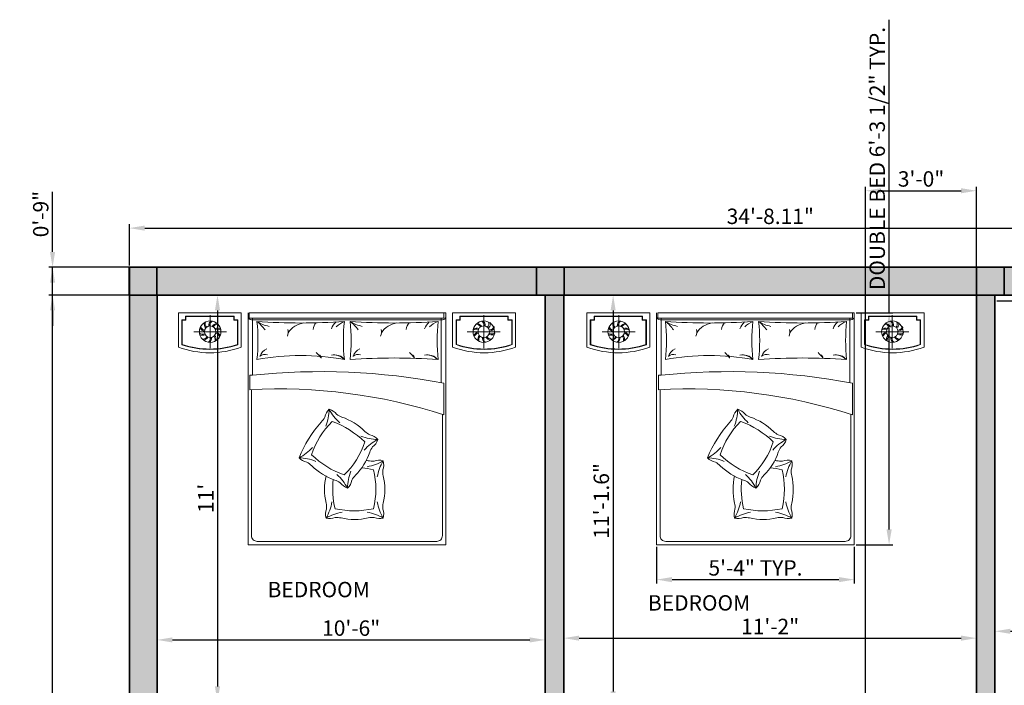
# Model space of a CAD drawing. Units: inches. Extents: x -36 to 490, y -420 to 94.
# Tile 3 of 4: x -36 to 284, y -122 to 94. Entities that reach past the tile are written whole.
import ezdxf

# ---------------------------------------------------------------- set-up
doc = ezdxf.new("R2010")
doc.units = ezdxf.units.IN
for name, color, linetype, lineweight in [('A-ANNO-DIMS', 2, 'Continuous', 18), ('A-AREA-IDEN', 1, 'Continuous', 18), ('A-COLS', 1, 'Continuous', 35), ('A-WALL', 7, 'Continuous', 35), ('furn', 8, 'Continuous', 18)]:
    doc.layers.add(name, color=color, linetype=linetype, lineweight=lineweight)
doc.layers.add('A-WALL-PATT', color=177, linetype='Continuous', lineweight=13, true_color=0x293189)
doc.styles.get("Standard").update_dxf_attribs({"font": 'arial.ttf'})
doc.dimstyles.new('ISO-25', dxfattribs={"dimtxt": 5, "dimasz": 5, "dimexe": 1.25, "dimexo": 0.625, "dimtad": 1, "dimlunit": 3, "dimtxsty": 'Standard', "dimcen": 2.5, "dimadec": 0, "dimazin": 0, "dimtfac": 1, "dimtmove": 0, "dimatfit": 3, "dimfxl": 1, "dimarcsym": 0})

# ---------------------------------------------------------------- blocks, each defined once
blk = doc.blocks.new('*D11')
at = {"layer": 'A-ANNO-DIMS', "color": 0, "lineweight": -2, "transparency": 16777216}
for p, q in [((8.98, -106.51), (8.98, -105.89)), ((13.98, -107.14), (129.98, -107.14)), ((134.98, -106.51), (134.98, -105.89))]:
    blk.add_line(p, q, dxfattribs=at)
at = {"layer": 'A-ANNO-DIMS', "color": 0, "transparency": 16777216}
for points in [[(13.98, -106.3), (13.98, -107.97), (8.98, -107.14)], [(129.98, -106.3), (129.98, -107.97), (134.98, -107.14)]]:
    blk.add_solid(points, dxfattribs=at)
at = {"layer": 'Defpoints', "color": 0, "transparency": 16777216}
for p in [(8.98, -107.14), (134.98, -107.14), (134.98, -107.14)]:
    blk.add_point(p, dxfattribs=at)
at = {"layer": 'A-ANNO-DIMS', "color": 0, "transparency": 16777216, "insert": (71.98, -103.96), "char_height": 5, "attachment_point": 5}
blk.add_mtext('10\'-6"', dxfattribs=at)
blk = doc.blocks.new('*D12')
at = {"layer": 'A-ANNO-DIMS', "color": 0, "lineweight": -2, "transparency": 16777216}
for p, q in [((9.61, 4.77), (29.84, 4.77)), ((28.59, -0.23), (28.59, -122.23)), ((9.61, -127.23), (29.84, -127.23))]:
    blk.add_line(p, q, dxfattribs=at)
at = {"layer": 'A-ANNO-DIMS', "color": 0, "transparency": 16777216}
for points in [[(27.76, -0.23), (29.43, -0.23), (28.59, 4.77)], [(27.76, -122.23), (29.43, -122.23), (28.59, -127.23)]]:
    blk.add_solid(points, dxfattribs=at)
at = {"layer": 'Defpoints', "color": 0, "transparency": 16777216}
for p in [(8.98, 4.77), (8.98, -127.23), (28.59, -127.23)]:
    blk.add_point(p, dxfattribs=at)
at = {"layer": 'A-ANNO-DIMS', "color": 0, "transparency": 16777216, "insert": (25.46, -61.23), "char_height": 5, "attachment_point": 5, "rotation": 90}
blk.add_mtext("11'", dxfattribs=at)
blk = doc.blocks.new('*D13')
at = {"layer": 'A-ANNO-DIMS', "color": 0, "lineweight": -2, "transparency": 16777216}
for p, q in [((140.98, -105.94), (140.98, -105.31)), ((274.98, -105.94), (274.98, -105.31)), ((145.98, -106.56), (269.98, -106.56))]:
    blk.add_line(p, q, dxfattribs=at)
at = {"layer": 'A-ANNO-DIMS', "color": 0, "transparency": 16777216}
for points in [[(145.98, -105.73), (145.98, -107.39), (140.98, -106.56)], [(269.98, -105.73), (269.98, -107.39), (274.98, -106.56)]]:
    blk.add_solid(points, dxfattribs=at)
at = {"layer": 'Defpoints', "color": 0, "transparency": 16777216}
for p in [(140.98, -106.56), (274.98, -106.56), (274.98, -106.56)]:
    blk.add_point(p, dxfattribs=at)
at = {"layer": 'A-ANNO-DIMS', "color": 0, "transparency": 16777216, "insert": (207.98, -103.42), "char_height": 5, "attachment_point": 5}
blk.add_mtext('11\'-2"', dxfattribs=at)
blk = doc.blocks.new('*D14')
at = {"layer": 'A-ANNO-DIMS', "color": 0, "lineweight": -2, "transparency": 16777216}
for p, q in [((141.61, 4.77), (158.28, 4.77)), ((157.03, -0.23), (157.03, -123.83)), ((143.3, -128.83), (158.28, -128.83))]:
    blk.add_line(p, q, dxfattribs=at)
at = {"layer": 'A-ANNO-DIMS', "color": 0, "transparency": 16777216}
for points in [[(156.2, -0.23), (157.86, -0.23), (157.03, 4.77)], [(156.2, -123.83), (157.86, -123.83), (157.03, -128.83)]]:
    blk.add_solid(points, dxfattribs=at)
at = {"layer": 'Defpoints', "color": 0, "transparency": 16777216}
for p in [(140.98, 4.77), (142.67, -128.83), (157.03, -128.83)]:
    blk.add_point(p, dxfattribs=at)
at = {"layer": 'A-ANNO-DIMS', "color": 0, "transparency": 16777216, "insert": (153.85, -62.03), "char_height": 5, "attachment_point": 5, "rotation": 90}
blk.add_mtext('11\'-1.6"', dxfattribs=at)
blk = doc.blocks.new('*D15')
at = {"layer": 'A-ANNO-DIMS', "color": 0, "lineweight": -2, "transparency": 16777216}
for p, q in [((281.61, 2.85), (295.66, 2.85)), ((294.41, -2.15), (294.41, -122.23)), ((281.61, -127.23), (295.66, -127.23))]:
    blk.add_line(p, q, dxfattribs=at)
at = {"layer": 'A-ANNO-DIMS', "color": 0, "transparency": 16777216}
for points in [[(293.58, -2.15), (295.25, -2.15), (294.41, 2.85)], [(293.58, -122.23), (295.25, -122.23), (294.41, -127.23)]]:
    blk.add_solid(points, dxfattribs=at)
at = {"layer": 'Defpoints', "color": 0, "transparency": 16777216}
for p in [(280.98, 2.85), (280.98, -127.23), (294.41, -127.23)]:
    blk.add_point(p, dxfattribs=at)
at = {"layer": 'A-ANNO-DIMS', "color": 0, "transparency": 16777216, "insert": (291.24, -62.19), "char_height": 5, "attachment_point": 5, "rotation": 90}
blk.add_mtext('10\'-10.08"', dxfattribs=at)
blk = doc.blocks.new('*D16')
at = {"layer": 'A-ANNO-DIMS', "color": 0, "lineweight": -2, "transparency": 16777216}
for p, q in [((280.98, -103.71), (280.98, -103.08)), ((285.98, -104.33), (401.98, -104.33)), ((406.98, -103.71), (406.98, -103.08))]:
    blk.add_line(p, q, dxfattribs=at)
at = {"layer": 'A-ANNO-DIMS', "color": 0, "transparency": 16777216}
for points in [[(285.98, -103.5), (285.98, -105.17), (280.98, -104.33)], [(401.98, -103.5), (401.98, -105.17), (406.98, -104.33)]]:
    blk.add_solid(points, dxfattribs=at)
at = {"layer": 'Defpoints', "color": 0, "transparency": 16777216}
for p in [(280.98, -104.33), (406.98, -104.33), (406.98, -104.33)]:
    blk.add_point(p, dxfattribs=at)
at = {"layer": 'A-ANNO-DIMS', "color": 0, "transparency": 16777216, "insert": (343.98, -101.16), "char_height": 5, "attachment_point": 5}
blk.add_mtext('10\'-6"', dxfattribs=at)
blk = doc.blocks.new('*D21')
at = {"layer": 'A-ANNO-DIMS', "color": 0, "lineweight": -2, "transparency": 16777216}
for p, q in [((-0.02, 14.4), (-0.02, 27.74)), ((4.98, 26.49), (411.1, 26.49)), ((416.1, 14.4), (416.1, 27.74))]:
    blk.add_line(p, q, dxfattribs=at)
at = {"layer": 'A-ANNO-DIMS', "color": 0, "transparency": 16777216}
for points in [[(4.98, 27.33), (4.98, 25.66), (-0.02, 26.49)], [(411.1, 27.33), (411.1, 25.66), (416.1, 26.49)]]:
    blk.add_solid(points, dxfattribs=at)
at = {"layer": 'Defpoints', "color": 0, "transparency": 16777216}
for p in [(416.1, 26.49), (-0.02, 13.77), (416.1, 13.77)]:
    blk.add_point(p, dxfattribs=at)
at = {"layer": 'A-ANNO-DIMS', "color": 0, "transparency": 16777216, "insert": (208.04, 29.67), "char_height": 5, "attachment_point": 5}
blk.add_mtext('34\'-8.11"', dxfattribs=at)
blk = doc.blocks.new('BED-DOUBLE')
for p, q in [((1.43, 73.57), (1.43, 55.04)), ((62.71, 73.57), (62.71, 52.63)), ((1.11, 73.01), (63.06, 73.01))]:
    blk.add_line(p, q)
for points in [[(0, 75.3), (0, 0), (64.18, 0), (64.18, 75.3)], [(63.58, 75.3), (63.58, 73.57), (0.37, 73.57), (0.37, 75.3), (64.18, 75.3)]]:
    blk.add_lwpolyline(points)
for points in [[(2.84, 60.1, 0.058596), (2.84, 72.5, 0.036889), (31.25, 72.5, 0.052163), (31.25, 60.1, 0.093111)], [(33.1, 60.1, 0.058596), (33.1, 72.5, 0.036648), (61.69, 72.5, 0.052163), (61.69, 60.1, 0.036967)], [(0.56, 55.04), (1.43, 55.04, -0.072944), (63.58, 52.45), (63.58, 42.16, 0.092568), (0.56, 50.32)]]:
    blk.add_lwpolyline(points, format="xyb", close=True)
for points in [[(1.11, 50.35), (1.11, 2.97, 0.414214), (2.97, 1.11), (61.21, 1.11, 0.414214), (63.06, 2.97), (63.06, 42.34)], [(25.2, 38.53, 0.091296), (26.33, 43.97, 0.091296), (29.75, 39.6, 0.091296)], [(20.61, 29.25, 0.111006), (31.2, 22.66, 0.119549), (37.88, 33.38, 0.107813), (27.32, 40)], [(27.26, 39.98, 0.121865), (20.61, 29.25, 0.121865)], [(36.64, 35.3, 0.091296), (42.07, 34.16, 0.091296), (37.69, 30.75, 0.091296)], [(32.26, 18.42, 0.159461), (33.7, 20.96, -0.076283), (34.84, 22.55, 0.115075), (39.49, 30.02, -0.076283), (40.42, 31.75, 0.159461), (42.07, 34.16)], [(21.95, 27.08, 0.091296), (16.52, 28.23, 0.091296), (20.9, 31.63, 0.091296)], [(38.64, 25.34, 0.091296), (43.86, 27.24, 0.091296), (41.94, 22.03, 0.091296)], [(43.86, 8.69, 0.159461), (43.73, 11.61, -0.076283), (43.86, 13.56, 0.115075), (43.86, 22.37, -0.076283), (43.73, 24.32, 0.159461), (43.86, 27.24)], [(28.24, 11.72, 0.111006), (40.71, 11.73, 0.119549), (40.71, 24.36, 0.033212), (36.88, 24.95)], [(33.39, 23.85, 0.091296), (32.26, 18.42, 0.091296), (28.84, 22.79)], [(30.52, 10.59, 0.091296), (25.31, 8.69, 0.091296), (27.23, 13.9, 0.091296)], [(41.94, 13.9, 0.091296), (43.86, 8.69, 0.091296), (38.64, 10.59)]]:
    blk.add_lwpolyline(points, format="xyb")
for centre, radius, start, end in [((1.11, 74.12), 1.11, 180, 270), ((63.06, 74.12), 1.11, 270, 0), ((9.44, 82.87), 12.28, 237.5379, 257.5233), ((-6.45, 60.91), 14.86, 36.4935, 51.2792), ((18.86, 65.15), 6.88, 96.6849, 148.3182), ((25.81, 69.06), 4.82, 141.8174, 169.8987), ((31.91, 68.38), 5.19, 130.5354, 160.3558), ((35.15, 64), 9.35, 114.6457, 134.1585), ((23.8, 60.91), 14.86, 36.4935, 51.2792), ((39.69, 82.87), 12.28, 237.5379, 257.5233), ((49.11, 65.15), 6.88, 96.6849, 148.3182), ((56.06, 69.06), 4.82, 141.8174, 169.8987), ((62.16, 68.38), 5.19, 130.5354, 160.3558), ((65.4, 64), 9.35, 114.6457, 134.1585), ((9.94, 68.98), 3.08, 335.8927, 16.1192), ((40.19, 68.98), 3.08, 335.8927, 16.1192), ((7.73, 59.82), 4.12, 114.2916, 160.9896), ((5.59, 58.96), 2.82, 76.4823, 128.5563), ((11.2, 51.48), 15.49, 36.2085, 45.0849), ((22.66, 60.63), 1.04, 353.7543, 77.2187), ((27.63, 56.56), 5.07, 44.406, 96.8342), ((28.58, 58.33), 3.21, 33.6349, 90.8456), ((37.98, 59.82), 4.12, 114.2916, 160.9896), ((35.84, 58.96), 2.82, 76.4823, 128.5563), ((41.46, 51.48), 15.49, 36.2085, 45.0849), ((52.91, 60.63), 1.04, 353.7543, 77.2187), ((57.88, 56.56), 5.07, 44.406, 96.8342), ((58.83, 58.33), 3.21, 33.6349, 90.8456), ((29.5, 40.5), 4.7, 132.4658, 168.7065), ((25.09, 39.6), 4.54, 37.2937, 74.0973), ((32.54, 47.52), 6.44, 233.2983, 250.7472), ((54.12, 12.85), 40.62, 138.3818, 157.7644), ((19.15, 44.34), 6.44, 315.5854, 333.0343), ((24.23, 23.07), 19.38, 45.1307, 71.3884), ((42.4, 41.42), 6.44, 225.7718, 243.2208), ((38.72, 31.4), 4.34, 39.4726, 79.6505), ((19.98, 31.41), 4.7, 222.6522, 258.8929), ((16.17, 21.05), 6.44, 45.7718, 63.2208), ((34.34, 39.4), 19.38, 225.1307, 251.3884), ((34.58, 8.4), 19.38, 77.0576, 78.7033), ((40.3, 33.58), 6.44, 257.6988, 275.1477), ((42.47, 23.13), 4.34, 71.3996, 111.5774), ((44.18, 17.97), 19.38, 166.8711, 193.1289), ((53.75, 18.1), 26.29, 173.1956, 194.0284), ((26.03, 14.95), 6.44, 53.2983, 70.7472), ((34.07, 23.48), 5.38, 218.7754, 250.3571), ((19.02, 12.17), 6.44, 355.0387, 12.4877), ((29.84, 9.96), 4.7, 159.3666, 195.6073), ((26.56, 13.23), 4.7, 254.5791, 290.8198), ((28.81, 2.42), 6.44, 77.6988, 95.1477), ((34.52, 27.6), 19.38, 257.0576, 283.3153), ((40.4, 2.45), 6.44, 85.2252, 102.6741), ((42.71, 13.95), 5.38, 250.7023, 282.284)]:
    blk.add_arc(centre, radius, start, end)
blk = doc.blocks.new('NIGHTSTAND-LAMP-L')
for p, q in [((10.31, 1.49), (10.31, 12.19)), ((4.96, 6.84), (15.66, 6.84))]:
    blk.add_line(p, q)
blk.add_lwpolyline([(0, 1.86), (0, 12.98), (20.4, 12.98), (20.4, 1.86, -0.181818)], format="xyb", close=True)
for points in [[(2.34, 11.87), (2.34, 10.65), (1.11, 10.65)], [(2.45, 11.87), (2.45, 10.54), (1.11, 10.54)], [(2.34, 11.87), (18.07, 11.87)], [(2.34, 11.76), (18.07, 11.76)], [(17.95, 11.87), (17.95, 10.54), (19.29, 10.54)], [(18.07, 11.87), (18.07, 10.65), (19.29, 10.65)]]:
    blk.add_lwpolyline(points)
for points in [[(19.29, 10.65), (19.29, 2.63, -0.167087), (1.11, 2.63), (1.11, 10.65)], [(19.18, 10.65), (19.18, 2.71, -0.165559), (1.22, 2.71), (1.22, 10.65)]]:
    blk.add_lwpolyline(points, format="xyb")
for radius in [3.49, 1.89]:
    blk.add_circle((10.31, 6.84), radius)
for centre, radius, start, end in [((10.62, 9.46), 2.24, 172.17, 218.4897), ((10.4, 9.41), 1.71, 160.3002, 220.538), ((12.1, 8.78), 2.24, 136.17, 182.4897), ((11.89, 8.87), 1.71, 124.3002, 184.538), ((9.02, 9.14), 2.24, 208.17, 254.4897), ((8.87, 8.97), 1.71, 196.3002, 256.538), ((12.89, 7.36), 2.24, 100.17, 146.4897), ((12.78, 7.55), 1.71, 88.3002, 148.538), ((12.7, 5.74), 2.24, 64.17, 110.4897), ((12.72, 5.96), 1.71, 52.3002, 112.538), ((11.59, 4.54), 2.24, 28.17, 74.4897), ((7.89, 7.72), 1.71, 232.3002, 292.538), ((7.91, 7.94), 2.24, 244.17, 290.4897), ((7.84, 6.13), 1.71, 268.3002, 328.538), ((7.72, 6.33), 2.24, 280.17, 326.4897), ((8.72, 4.82), 1.71, 304.3002, 4.538), ((8.52, 4.9), 2.24, 316.17, 2.4897), ((10.22, 4.27), 1.71, 340.3002, 40.538), ((10, 4.22), 2.24, 352.17, 38.4897), ((11.74, 4.71), 1.71, 16.3002, 76.538)]:
    blk.add_arc(centre, radius, start, end)
blk = doc.blocks.new('NIGHTSTAND-LAMP-R')
for p, q in [((10.1, 1.49), (10.1, 12.18)), ((15.45, 6.83), (4.75, 6.83))]:
    blk.add_line(p, q)
blk.add_lwpolyline([(20.4, 1.85), (20.4, 12.98), (0, 12.98), (0, 1.85, 0.181818)], format="xyb", close=True)
for points in [[(2.34, 11.87), (2.34, 10.65), (1.11, 10.65)], [(2.45, 11.87), (2.45, 10.53), (1.11, 10.53)], [(18.07, 11.87), (2.34, 11.87)], [(18.07, 11.76), (2.34, 11.76)], [(17.95, 11.87), (17.95, 10.53), (19.29, 10.53)], [(18.07, 11.87), (18.07, 10.65), (19.29, 10.65)]]:
    blk.add_lwpolyline(points)
for points in [[(1.11, 10.65), (1.11, 2.63, 0.167087), (19.29, 2.63), (19.29, 10.65)], [(1.22, 10.65), (1.22, 2.71, 0.165559), (19.18, 2.71), (19.18, 10.65)]]:
    blk.add_lwpolyline(points, format="xyb")
for radius in [3.49, 1.89]:
    blk.add_circle((10.1, 6.83), radius)
for centre, radius, start, end in [((8.51, 8.86), 1.71, 355.462, 55.6998), ((8.31, 8.77), 2.24, 357.5103, 43.83), ((10.01, 9.4), 1.71, 319.462, 19.6998), ((10.04, 9.55), 2.24, 321.5103, 7.83), ((7.68, 5.95), 1.71, 67.462, 127.6998), ((7.7, 5.73), 2.24, 69.5103, 115.83), ((8.81, 4.54), 2.24, 105.5103, 151.83), ((7.62, 7.54), 1.71, 31.462, 91.6998), ((7.51, 7.35), 2.24, 33.5103, 79.83), ((12.77, 7.81), 1.71, 247.462, 307.6998), ((11.79, 9.06), 1.71, 283.462, 343.6998), ((11.64, 9.23), 2.24, 285.5103, 331.83), ((8.66, 4.7), 1.71, 103.462, 163.6998), ((10.41, 4.22), 2.24, 141.5103, 187.83), ((10.19, 4.27), 1.71, 139.462, 199.6998), ((11.88, 4.9), 2.24, 177.5103, 223.83), ((11.68, 4.81), 1.71, 175.462, 235.6998), ((12.68, 6.32), 2.24, 213.5103, 259.83), ((12.57, 6.13), 1.71, 211.462, 271.6998), ((12.74, 8.03), 2.24, 249.5103, 295.83)]:
    blk.add_arc(centre, radius, start, end)
blk = doc.blocks.new('COLUMN-9X9')
h = blk.add_hatch(color=256)
h.dxf.hatch_style = 1
h.paths.add_polyline_path([(9, 0), (9, 9), (0, 9), (0, 0)])
blk.add_lwpolyline([(0, 9), (9, 9), (9, 0), (0, 0)], close=True)
blk = doc.blocks.new('*D30')
at = {"layer": 'A-ANNO-DIMS', "color": 0, "lineweight": -2, "transparency": 16777216}
for p, q in [((246.61, -0.97), (246.61, 94.12)), ((235.94, -0.97), (247.86, -0.97)), ((246.61, -71.28), (246.61, -5.97)), ((235.94, -76.28), (247.86, -76.28))]:
    blk.add_line(p, q, dxfattribs=at)
at = {"layer": 'A-ANNO-DIMS', "color": 0, "transparency": 16777216}
for points in [[(245.78, -5.97), (247.45, -5.97), (246.61, -0.97)], [(245.78, -71.28), (247.45, -71.28), (246.61, -76.28)]]:
    blk.add_solid(points, dxfattribs=at)
at = {"layer": 'Defpoints', "color": 0, "transparency": 16777216}
for p in [(235.32, -0.97), (246.61, -0.97), (235.32, -76.28)]:
    blk.add_point(p, dxfattribs=at)
at = {"layer": 'A-ANNO-DIMS', "color": 0, "transparency": 16777216, "insert": (243.4, 49.07), "char_height": 5, "attachment_point": 5, "rotation": 90}
blk.add_mtext('DOUBLE BED 6\'-3 1/2" TYP.', dxfattribs=at)
blk = doc.blocks.new('*D31')
at = {"layer": 'A-ANNO-DIMS', "color": 0, "lineweight": -2, "transparency": 16777216}
for p, q in [((171.14, -76.9), (171.14, -88.82)), ((235.32, -76.9), (235.32, -88.82)), ((176.14, -87.57), (230.32, -87.57))]:
    blk.add_line(p, q, dxfattribs=at)
at = {"layer": 'A-ANNO-DIMS', "color": 0, "transparency": 16777216}
for points in [[(176.14, -86.74), (176.14, -88.41), (171.14, -87.57)], [(230.32, -86.74), (230.32, -88.41), (235.32, -87.57)]]:
    blk.add_solid(points, dxfattribs=at)
at = {"layer": 'Defpoints', "color": 0, "transparency": 16777216}
for p in [(171.14, -76.28), (235.32, -76.28), (235.32, -87.57)]:
    blk.add_point(p, dxfattribs=at)
at = {"layer": 'A-ANNO-DIMS', "color": 0, "transparency": 16777216, "insert": (203.23, -84.41), "char_height": 5, "attachment_point": 5}
blk.add_mtext('5\'-4" TYP.', dxfattribs=at)
blk = doc.blocks.new('*D39')
at = {"layer": 'A-ANNO-DIMS', "color": 0, "lineweight": -2, "transparency": 16777216}
for p, q in [((238.98, -244.38), (238.98, 39.87)), ((243.98, 38.62), (269.98, 38.62)), ((274.98, -244.38), (274.98, 39.87))]:
    blk.add_line(p, q, dxfattribs=at)
at = {"layer": 'A-ANNO-DIMS', "color": 0, "transparency": 16777216}
for points in [[(243.98, 39.45), (243.98, 37.79), (238.98, 38.62)], [(269.98, 39.45), (269.98, 37.79), (274.98, 38.62)]]:
    blk.add_solid(points, dxfattribs=at)
at = {"layer": 'Defpoints', "color": 0, "transparency": 16777216}
for p in [(274.98, 38.62), (238.98, -245.01), (274.98, -245.01)]:
    blk.add_point(p, dxfattribs=at)
at = {"layer": 'A-ANNO-DIMS', "color": 0, "transparency": 16777216, "insert": (256.98, 41.8), "char_height": 5, "attachment_point": 5}
blk.add_mtext('3\'-0"', dxfattribs=at)
blk = doc.blocks.new('*D42')
at = {"layer": 'A-ANNO-DIMS', "color": 0, "lineweight": -2, "transparency": 16777216}
for p, q in [((-0.64, 13.77), (-26.2, 13.77)), ((-24.95, -385.69), (-24.95, 8.77)), ((140.36, -390.69), (-26.2, -390.69))]:
    blk.add_line(p, q, dxfattribs=at)
at = {"layer": 'A-ANNO-DIMS', "color": 0, "transparency": 16777216}
for points in [[(-25.78, 8.77), (-24.12, 8.77), (-24.95, 13.77)], [(-25.78, -385.69), (-24.12, -385.69), (-24.95, -390.69)]]:
    blk.add_solid(points, dxfattribs=at)
at = {"layer": 'Defpoints', "color": 0, "transparency": 16777216}
for p in [(-24.95, 13.77), (-0.02, 13.77), (140.98, -390.69)]:
    blk.add_point(p, dxfattribs=at)
at = {"layer": 'A-ANNO-DIMS', "color": 0, "transparency": 16777216, "insert": (-28.16, -188.46), "char_height": 5, "attachment_point": 5, "rotation": 90}
blk.add_mtext('33\'-8 1/2"', dxfattribs=at)
blk = doc.blocks.new('*D50')
at = {"layer": 'A-ANNO-DIMS', "color": 0, "lineweight": -2, "transparency": 16777216}
for p, q in [((-24.95, 18.77), (-24.95, 38.31)), ((8.28, 13.77), (-26.2, 13.77)), ((-24.95, 4.77), (-24.95, 13.77)), ((8.36, 4.77), (-26.2, 4.77)), ((-24.95, -0.23), (-24.95, -5.23))]:
    blk.add_line(p, q, dxfattribs=at)
at = {"layer": 'A-ANNO-DIMS', "color": 0, "transparency": 16777216}
for points in [[(-25.78, 18.77), (-24.12, 18.77), (-24.95, 13.77)], [(-25.78, -0.23), (-24.12, -0.23), (-24.95, 4.77)]]:
    blk.add_solid(points, dxfattribs=at)
at = {"layer": 'Defpoints', "color": 0, "transparency": 16777216}
for p in [(-24.95, 13.77), (8.9, 13.77), (8.98, 4.77)]:
    blk.add_point(p, dxfattribs=at)
at = {"layer": 'A-ANNO-DIMS', "color": 0, "transparency": 16777216, "insert": (-28.13, 31.04), "char_height": 5, "attachment_point": 5, "rotation": 90}
blk.add_mtext('0\'-9"', dxfattribs=at)

msp = doc.modelspace()

# ---------------------------------------------------------------- hatches: boundary and pattern name
at = {"layer": 'A-WALL-PATT'}
h = msp.add_hatch(color=256, dxfattribs=at)
h.dxf.hatch_style = 1
h.paths.add_polyline_path([(132.114, 13.772), (8.901, 13.772), (8.901, 4.772), (132.114, 4.772)])
h.paths.add_polyline_path([(274.98, 13.772), (141.114, 13.772), (141.114, 4.772), (274.98, 4.772)])
h.paths.add_polyline_path([(407.097, 13.772), (283.98, 13.772), (283.98, 4.772), (407.097, 4.772)])
h.paths.add_polyline_path([(280.984, 4.772), (274.984, 4.772), (274.984, -127.228), (280.984, -127.228)])
h.paths.add_polyline_path([(274.984, -127.228), (176.984, -127.228), (176.984, -133.228), (274.984, -133.228)])
h.paths.add_polyline_path([(140.984, 4.772), (134.984, 4.772), (134.984, -128.829), (140.984, -128.829)])
h.paths.add_polyline_path([(8.984, 4.772), (8.901, 4.772), (-0.016, 4.772), (-0.016, -127.003), (8.984, -127.003)])
h.paths.add_polyline_path([(94.984, -127.228), (8.984, -127.228), (8.984, -133.228), (88.984, -133.228), (88.984, -151.228), (94.984, -151.228), (94.984, -133.228)])
h.paths.add_polyline_path([(8.984, -136.003), (-0.016, -136.003), (-0.016, -228.965), (8.984, -228.965)])
h.paths.add_polyline_path([(100.984, -181.228), (98.984, -181.228), (88.984, -181.228), (8.984, -181.228), (8.984, -187.228), (88.984, -187.228), (94.984, -187.228), (94.984, -235.228), (134.793, -235.228), (134.793, -229.228), (100.984, -229.228)])
h.paths.add_polyline_path([(64.984, -229.228), (9.003, -229.228), (9.003, -235.228), (64.984, -235.228)], flags=17)
h.paths.add_polyline_path([(8.984, -237.965), (-0.016, -237.965), (-0.016, -366.285), (8.984, -366.285)])
h.paths.add_polyline_path([(132.054, -366.228), (9.018, -366.228), (9.018, -375.228), (132.054, -375.228)])
h.paths.add_polyline_path([(140.984, -271.228), (134.984, -271.228), (134.984, -366.131), (140.984, -366.131)])

# ---------------------------------------------------------------- linework, layer by layer
at = {"layer": 'A-WALL'}
for p, q in [((8.984, 4.772), (134.984, 4.772)), ((8.984, -366.228), (8.984, 4.772)), ((134.984, -133.228), (134.984, 4.772)), ((140.984, 4.772), (274.984, 4.772)), ((140.984, -133.228), (140.984, 4.772)), ((274.984, -366.228), (274.984, 4.772)), ((280.984, -366.228), (280.984, 4.772)), ((280.984, 4.772), (406.984, 4.772))]:
    msp.add_line(p, q, dxfattribs=at)
msp.add_lwpolyline([(-0.016, 13.772), (415.984, 13.772), (415.984, -375.228), (-0.016, -375.228)], close=True, dxfattribs=at)

# ---------------------------------------------------------------- block references
at = {"layer": 'A-COLS'}
for p, rotation in [((-0.099, 13.772), 269.9999999999997), ((132.113, 13.772), 269.9999999999995), ((274.98, 13.772), 269.9999999999993)]:
    msp.add_blockref('COLUMN-9X9', p, dxfattribs=dict(at, rotation=rotation))
at = {"layer": 'furn'}
for name, p in [('NIGHTSTAND-LAMP-L', (15.906, -13.963)), ('BED-DOUBLE', (38.534, -76.278)), ('NIGHTSTAND-LAMP-R', (104.935, -13.958)), ('NIGHTSTAND-LAMP-L', (148.514, -13.963)), ('BED-DOUBLE', (171.142, -76.278)), ('NIGHTSTAND-LAMP-R', (237.543, -13.958))]:
    msp.add_blockref(name, p, dxfattribs=at)

# ---------------------------------------------------------------- texts
at = {"layer": 'A-AREA-IDEN', "char_height": 5, "attachment_point": 1}
for width, insert in [(72.65081, (44.844, -88.298)), (74.62994, (168.325, -92.616))]:
    msp.add_mtext_dynamic_manual_height_columns('{BEDROOM}', width=width, gutter_width=12.5, heights=[0], dxfattribs=dict(at, insert=insert))

# ---------------------------------------------------------------- dimensions: what is measured, and where the dimension line sits
at = {"layer": 'A-ANNO-DIMS'}
dim = msp.add_linear_dim(base=(246.613, -0.974), p1=(235.318, -76.278), p2=(235.318, -0.974), angle=90, text='DOUBLE BED <> TYP.', dimstyle='ISO-25', override={"dimdec": 1, "dimlfac": 1, "dimrnd": 0, "dimzin": 1, "dimdsep": 46, "dimlunit": 4, "dimfrac": 2}, dxfattribs=at)
dim.commit()
dim.dimension.update_dxf_attribs({"geometry": '*D30', "text_midpoint": (243.4, 49.075)})
for base, p1, p2, override, picture, middle in [((274.984, 38.622), (238.984, -245.007), (274.984, -245.007), {"dimdec": 1, "dimlfac": 1, "dimrnd": 0, "dimzin": 1, "dimdsep": 46, "dimlunit": 4, "dimfrac": 2}, '*D39', (256.984, 41.801)), ((416.097, 26.492), (-0.016, 13.772), (416.097, 13.772), {"dimclrd": 0, "dimclre": 0, "dimclrt": 0}, '*D21', (208.04, 29.671)), ((406.984, -104.334), (280.984, -104.334), (406.984, -104.334), {"dimclrd": 0, "dimclre": 0, "dimclrt": 0}, '*D16', (343.984, -101.156)), ((134.984, -107.136), (8.984, -107.136), (134.984, -107.136), {"dimclrd": 0, "dimclre": 0, "dimclrt": 0}, '*D11', (71.984, -103.958)), ((274.984, -106.56), (140.984, -106.56), (274.984, -106.56), {"dimclrd": 0, "dimclre": 0, "dimclrt": 0}, '*D13', (207.984, -103.425))]:
    dim = msp.add_linear_dim(base=base, p1=p1, p2=p2, dimstyle='ISO-25', override=override, dxfattribs=at)
    dim.commit()
    dim.dimension.update_dxf_attribs({"geometry": picture, "text_midpoint": middle})
for base, p1, p2, override, picture, middle in [((-24.949, 13.772), (8.984, 4.772), (8.901, 13.772), {"dimdec": 1, "dimlfac": 1, "dimrnd": 0, "dimzin": 1, "dimdsep": 46, "dimlunit": 4, "dimfrac": 2}, '*D50', (-28.126, 31.042)), ((-24.949, 13.772), (140.984, -390.685), (-0.016, 13.772), {"dimdec": 1, "dimlfac": 1, "dimrnd": 0, "dimzin": 1, "dimdsep": 46, "dimlunit": 4, "dimfrac": 2}, '*D42', (-28.161, -188.457)), ((28.594, -127.228), (8.984, 4.772), (8.984, -127.228), {"dimclrd": 0, "dimclre": 0, "dimclrt": 0}, '*D12', (25.459, -61.228)), ((157.031, -128.829), (140.984, 4.772), (142.675, -128.829), {"dimclrd": 0, "dimclre": 0, "dimclrt": 0}, '*D14', (153.853, -62.029)), ((294.414, -127.228), (280.984, 2.849), (280.984, -127.228), {"dimclrd": 0, "dimclre": 0, "dimclrt": 0}, '*D15', (291.236, -62.19))]:
    dim = msp.add_linear_dim(base=base, p1=p1, p2=p2, angle=90, dimstyle='ISO-25', override=override, dxfattribs=at)
    dim.commit()
    dim.dimension.update_dxf_attribs({"geometry": picture, "text_midpoint": middle})
dim = msp.add_linear_dim(base=(235.318, -87.573), p1=(171.142, -76.278), p2=(235.318, -76.278), text='<> TYP.', dimstyle='ISO-25', override={"dimdec": 1, "dimlfac": 1, "dimrnd": 0, "dimzin": 1, "dimdsep": 46, "dimlunit": 4, "dimfrac": 2}, dxfattribs=at)
dim.commit()
dim.dimension.update_dxf_attribs({"geometry": '*D31', "text_midpoint": (203.23, -84.406)})

doc.saveas('drawing.dxf')
